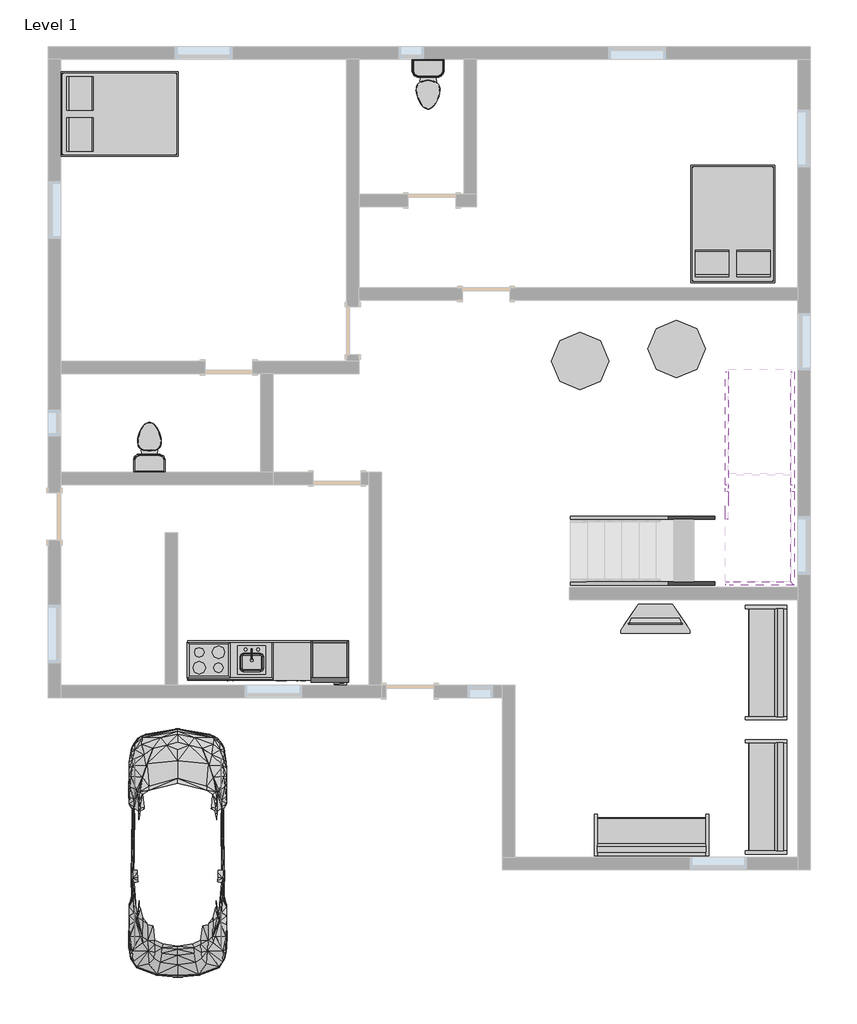
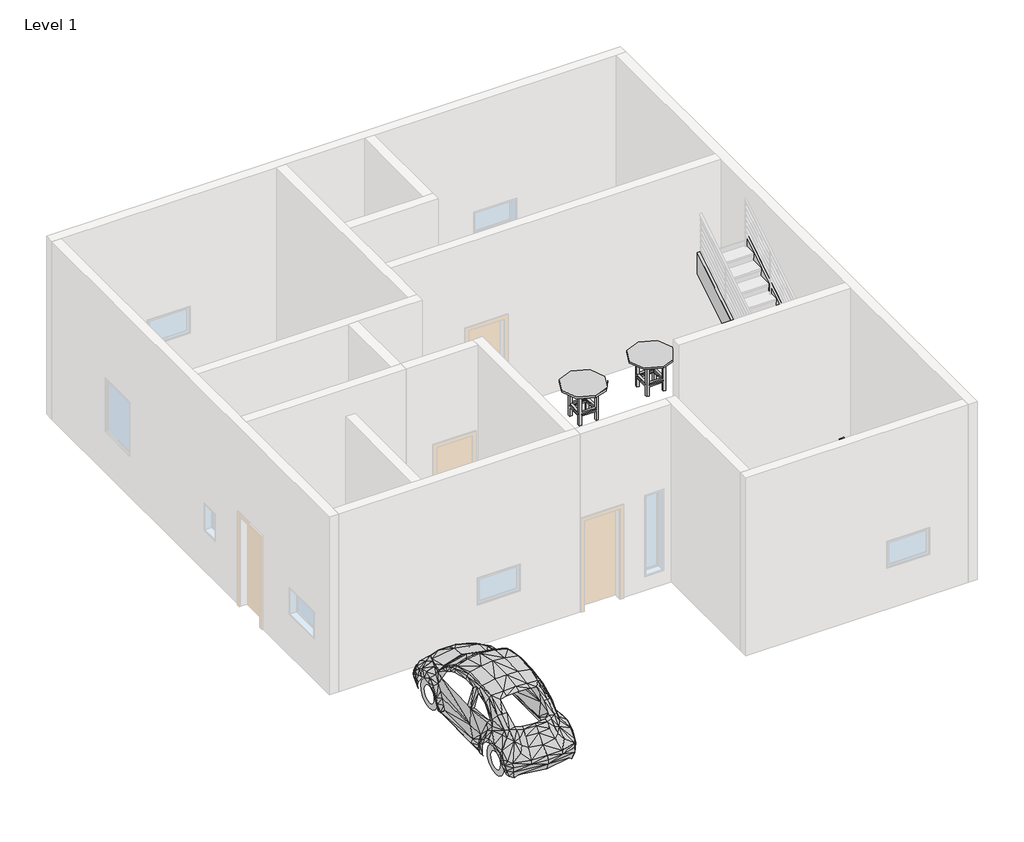
# One storey, part 4 of 4: 10 furniture elements, 7 members, 5 proxies, 3 flow terminals.
"""IFC4 building model written with IfcOpenShell, lengths in millimetres."""

from ifc_helpers import new_model, si_unit, frame, origin, place, context, project, spatial, polyline, outline, extrude, faceted_brep, transform, mapped, element, save
from components import m_cook_top_4_unit2_0615_x_500mm_249f3515, m_dishwasher_610_x_610_x_875mm_54ecfc4c, m_kitchenette_medium_1372mm_e05c6bec, m_rpc_beetle_m_rpc_beetle_b6d71803, m_refrigerator_600_x_660mm_a466bf94, m_sink_kitchen_island_450_x_450mm_f969cf2d, m_toilet_domestic_3d_m_toilet_domestic_3d_5cb52bd4, m_toilet_domestic_3d_m_toilet_domestic_3d_183bbd19, furniture_40ec15d9, furniture_0810mm_56245f3a, m_bed_box_1346_x_1880mm_double_b32eb57e, m_counter_top_w_sink_hole_600mm_depth_0a237b63, m_sofa_1830mm_f9e8a66b, m_table_dining_round_w_chairs_0915mm_diameter_5defa876

model = new_model("IFC4")

# Units and contexts
model_context = context("Model", 3, world=origin())
ifc_project = project(units=[si_unit("LENGTHUNIT", "METRE", prefix="MILLI")], contexts=[model_context])

# Site, building, storey
site = spatial("IfcSite", under=ifc_project)
building = spatial("IfcBuilding", under=site)
storey = spatial("IfcBuildingStorey", under=building, Name="Level 1", Elevation=0.0)

# Proxies
placement = place(None, origin())
m_cook_top_4_unit2_0615_x_500mm_shape = m_cook_top_4_unit2_0615_x_500mm_249f3515(model_context)
element("IfcBuildingElementProxy", 1, Name="M_Cook Top-4 Unit2 : 0615 x 500mm", ObjectType="M_Cook Top-4 Unit2 : 0615 x 500mm", at=placement, inside=storey, context=model_context, shape_type="MappedRepresentation", body=[
    mapped(m_cook_top_4_unit2_0615_x_500mm_shape, transform((-6183.3732634, 1498.698464, 0.0), x_axis=(1.0, 0.0, 0.0), y_axis=(0.0, 1.0, 0.0), z_axis=(0.0, 0.0, 1.0))),
])
m_dishwasher_610_x_610_x_875mm_shape = m_dishwasher_610_x_610_x_875mm_54ecfc4c(model_context)
element("IfcBuildingElementProxy", 2, Name="M_Dishwasher : 610 x 610 x 875mm", ObjectType="M_Dishwasher : 610 x 610 x 875mm", at=placement, inside=storey, context=model_context, shape_type="MappedRepresentation", body=[
    mapped(m_dishwasher_610_x_610_x_875mm_shape, transform((-5233.8907319, 1232.0488992, 0.0), x_axis=(1.0, 0.0, 0.0), y_axis=(0.0, 1.0, 0.0), z_axis=(0.0, 0.0, 1.0))),
])
m_kitchenette_medium_1372mm_shape = m_kitchenette_medium_1372mm_e05c6bec(model_context)
element("IfcBuildingElementProxy", 3, Name="M_Kitchenette - Medium : 1372mm", ObjectType="M_Kitchenette - Medium : 1372mm", at=placement, inside=storey, context=model_context, shape_type="MappedRepresentation", body=[
    mapped(m_kitchenette_medium_1372mm_shape, transform((-5859.1109683, 1803.698464, 0.0), x_axis=(1.0, 0.0, 0.0), y_axis=(0.0, 1.0, 0.0), z_axis=(0.0, 0.0, 1.0))),
])
m_rpc_beetle_m_rpc_beetle_shape = m_rpc_beetle_m_rpc_beetle_b6d71803(model_context)
element("IfcBuildingElementProxy", 4, Name="M_RPC Beetle : M_RPC Beetle", ObjectType="M_RPC Beetle : M_RPC Beetle", at=placement, inside=storey, context=model_context, shape_type="MappedRepresentation", body=[
    mapped(m_rpc_beetle_m_rpc_beetle_shape, transform((-6679.9732634, -2820.751536, 0.0), x_axis=(1.0, 0.0, 0.0), y_axis=(0.0, 1.0, 0.0), z_axis=(0.0, 0.0, 1.0))),
])
m_refrigerator_600_x_660mm_shape = m_refrigerator_600_x_660mm_a466bf94(model_context)
element("IfcBuildingElementProxy", 5, Name="M_Refrigerator : 600 x 660mm", ObjectType="M_Refrigerator : 600 x 660mm", at=placement, inside=storey, context=model_context, shape_type="MappedRepresentation", body=[
    mapped(m_refrigerator_600_x_660mm_shape, transform((-4192.5721207, 1507.4833738, 0.0), x_axis=(1.0, 0.0, 0.0), y_axis=(0.0, 1.0, 0.0), z_axis=(0.0, 0.0, 1.0))),
])

# Flow terminals
m_sink_kitchen_island_450_x_450mm_shape = m_sink_kitchen_island_450_x_450mm_f969cf2d(model_context)
element("IfcFlowTerminal", 6, ObjectType="M_Sink Kitchen-Island : 450 x 450mm", at=placement, inside=storey, context=model_context, shape_type="MappedRepresentation", body=[
    mapped(m_sink_kitchen_island_450_x_450mm_shape, transform((-5513.062504, 1496.3530629, 0.0), x_axis=(1.0, 0.0, 0.0), y_axis=(0.0, 1.0, 0.0), z_axis=(0.0, 0.0, 1.0))),
])
m_toilet_domestic_3d_m_toilet_domestic_3d_shape = m_toilet_domestic_3d_m_toilet_domestic_3d_5cb52bd4(model_context)
m_toilet_domestic_3d_m_toilet_domestic_3d_2_shape = m_toilet_domestic_3d_m_toilet_domestic_3d_183bbd19(model_context)
element("IfcFlowTerminal", 7, ObjectType="M_Toilet-Domestic-3D : M_Toilet-Domestic-3D", at=placement, inside=storey, context=model_context, shape_type="MappedRepresentation", body=[
    mapped(m_toilet_domestic_3d_m_toilet_domestic_3d_shape, transform((-7133.3692907, 4995.5444913, 0.0), x_axis=(-1.0, 0.0, 0.0), y_axis=(0.0, -1.0, 0.0), z_axis=(0.0, 0.0, 1.0))),
    mapped(m_toilet_domestic_3d_m_toilet_domestic_3d_2_shape, transform((-7133.3692907, 4995.5444913, 0.0), x_axis=(-1.0, 0.0, 0.0), y_axis=(0.0, -1.0, 0.0), z_axis=(0.0, 0.0, 1.0))),
])
element("IfcFlowTerminal", 8, ObjectType="M_Toilet-Domestic-3D : M_Toilet-Domestic-3D", at=placement, inside=storey, context=model_context, shape_type="MappedRepresentation", body=[
    mapped(m_toilet_domestic_3d_m_toilet_domestic_3d_shape, transform((-2677.5646035, 10610.1524366, 0.0), x_axis=(1.0, 0.0, 0.0), y_axis=(0.0, 1.0, 0.0), z_axis=(0.0, 0.0, 1.0))),
    mapped(m_toilet_domestic_3d_m_toilet_domestic_3d_2_shape, transform((-2677.5646035, 10610.1524366, 0.0), x_axis=(1.0, 0.0, 0.0), y_axis=(0.0, 1.0, 0.0), z_axis=(0.0, 0.0, 1.0))),
])

# Furniture
furniture_shape = furniture_40ec15d9(model_context)
element("IfcFurniture", 9, at=placement, inside=storey, context=model_context, shape_type="MappedRepresentation", body=[
    mapped(furniture_shape, transform((832.4258439, 2387.898464, 0.0), x_axis=(1.0, 0.0, 0.0), y_axis=(0.0, 1.0, 0.0), z_axis=(0.0, 0.0, 1.0))),
])
furniture_0810mm_shape = furniture_0810mm_56245f3a(model_context)
element("IfcFurniture", 10, ObjectType="0810mm", at=placement, inside=storey, context=model_context, shape_type="MappedRepresentation", body=[
    mapped(furniture_0810mm_shape, transform((961.5583601, 2138.8495806, 0.0), x_axis=(1.0, 0.0, 0.0), y_axis=(0.0, 1.0, 0.0), z_axis=(0.0, 0.0, 1.0))),
])
m_bed_box_1346_x_1880mm_double_shape = m_bed_box_1346_x_1880mm_double_b32eb57e(model_context)
element("IfcFurniture", 11, ObjectType="M_Bed-Box : 1346 x 1880mm - Double", at=placement, inside=storey, context=model_context, shape_type="MappedRepresentation", body=[
    mapped(m_bed_box_1346_x_1880mm_double_shape, transform((-7849.2027716, 9887.896005, 0.0), x_axis=(0.0, 1.0, 0.0), y_axis=(-1.0, 0.0, 0.0), z_axis=(0.0, 0.0, 1.0))),
])
element("IfcFurniture", 12, ObjectType="M_Bed-Box : 1346 x 1880mm - Double", at=placement, inside=storey, context=model_context, shape_type="MappedRepresentation", body=[
    mapped(m_bed_box_1346_x_1880mm_double_shape, transform((2536.3791956, 8233.0189558, 0.0), x_axis=(-1.0, 0.0, 0.0), y_axis=(0.0, -1.0, 0.0), z_axis=(0.0, 0.0, 1.0))),
])
m_counter_top_w_sink_hole_600mm_depth_shape = m_counter_top_w_sink_hole_600mm_depth_0a237b63(model_context)
element("IfcFurniture", 13, ObjectType="M_Counter Top w Sink Hole : 600mm Depth", at=placement, inside=storey, context=model_context, shape_type="MappedRepresentation", body=[
    mapped(m_counter_top_w_sink_hole_600mm_depth_shape, transform((-5325.9109683, 1803.698464, 0.0), x_axis=(1.0, 0.0, 0.0), y_axis=(0.0, 1.0, 0.0), z_axis=(0.0, 0.0, 1.0))),
])
m_sofa_1830mm_shape = m_sofa_1830mm_f9e8a66b(model_context)
element("IfcFurniture", 14, ObjectType="M_Sofa : 1830mm", at=placement, inside=storey, context=model_context, shape_type="MappedRepresentation", body=[
    mapped(m_sofa_1830mm_shape, transform((2581.4726382, 1526.4189558, 0.0), x_axis=(0.0, -0.9999999999999999, 0.0), y_axis=(0.9999999999999999, 0.0, 0.0), z_axis=(0.0, 0.0, 1.0))),
])
element("IfcFurniture", 15, ObjectType="M_Sofa : 1830mm", at=placement, inside=storey, context=model_context, shape_type="MappedRepresentation", body=[
    mapped(m_sofa_1830mm_shape, transform((2581.4726382, -616.7810442, 0.0), x_axis=(0.0, -1.0, 0.0), y_axis=(1.0, 0.0, 0.0), z_axis=(0.0, 0.0, 1.0))),
])
element("IfcFurniture", 16, ObjectType="M_Sofa : 1830mm", at=placement, inside=storey, context=model_context, shape_type="MappedRepresentation", body=[
    mapped(m_sofa_1830mm_shape, transform((969.1972284, -1150.5974377, 0.0), x_axis=(-1.0000000000000004, 0.0, 0.0), y_axis=(0.0, -1.0000000000000004, 0.0), z_axis=(0.0, 0.0, 1.0))),
])
m_table_dining_round_w_chairs_0915mm_diameter_shape = m_table_dining_round_w_chairs_0915mm_diameter_5defa876(model_context)
element("IfcFurniture", 17, ObjectType="M_Table-Dining Round w Chairs : 0915mm Diameter", at=placement, inside=storey, context=model_context, shape_type="MappedRepresentation", body=[
    mapped(m_table_dining_round_w_chairs_0915mm_diameter_shape, transform((-349.4250983, 6462.1271525, 0.0), x_axis=(1.0, 0.0, 0.0), y_axis=(0.0, 1.0, 0.0), z_axis=(0.0, 0.0, 1.0))),
])
element("IfcFurniture", 18, ObjectType="M_Table-Dining Round w Chairs : 0915mm Diameter", at=placement, inside=storey, context=model_context, shape_type="MappedRepresentation", body=[
    mapped(m_table_dining_round_w_chairs_0915mm_diameter_shape, transform((1193.5913431, 6656.0887971, 0.0), x_axis=(1.0, 0.0, 0.0), y_axis=(0.0, 1.0, 0.0), z_axis=(0.0, 0.0, 1.0))),
])

# Members
element("IfcMember", 19, ObjectType="Stringer - 50mm Width", at=placement, inside=storey, context=model_context, shape_type="SweptSolid", body=[
    extrude(outline(polyline([(215.089535, -399.786154), (0.0, -399.786154), (0.0, 8.4725788), (1307.5359792, 2076.013846), (1780.8128552, 2076.013846), (215.089535, -399.786154)])), frame((0.0, 3747.052048, 0.0), z_axis=(0.0, 1.0, 0.0), x_axis=(0.0, 0.0, 1.0)), (0.0, 0.0, 1.0), 50.0),
])
element("IfcMember", 20, ObjectType="Stringer - 50mm Width", at=placement, inside=storey, context=model_context, shape_type="SweptSolid", body=[
    extrude(outline(polyline([(215.089535, -399.786154), (0.0, -399.786154), (0.0, 8.4725788), (1386.5241617, 2200.9139095), (1786.5241617, 2085.0448495), (215.089535, -399.786154)])), frame((0.0, 2697.0262668, 0.0), z_axis=(0.0, 1.0, 0.0), x_axis=(0.0, 0.0, 1.0)), (0.0, 0.0, 1.0), 50.0),
])
element("IfcMember", 21, ObjectType="Stringer - 50mm Width", at=placement, inside=storey, context=model_context, shape_type="SweptSolid", body=[
    extrude(outline(polyline([(4303.9485275, 1386.5241617), (4188.0794675, 1786.5241617), (6103.248464, 2997.6982306), (6103.248464, 2524.4213547), (4303.9485275, 1386.5241617)])), frame((2076.013846, 0.0, 0.0), z_axis=(1.0, 0.0, 0.0), x_axis=(0.0, 1.0, 0.0)), (0.0, 0.0, 1.0), 50.0),
])
element("IfcMember", 22, ObjectType="Stringer - 50mm Width", at=placement, inside=storey, context=model_context, shape_type="SweptSolid", body=[
    extrude(outline(polyline([(4303.9485275, 1386.5241617), (4188.0794675, 1786.5241617), (6103.248464, 2997.6982306), (6103.248464, 2524.4213547), (4303.9485275, 1386.5241617)])), frame((3126.0396272, 0.0, 0.0), z_axis=(1.0, 0.0, 0.0), x_axis=(0.0, 1.0, 0.0)), (0.0, 0.0, 1.0), 50.0),
])
element("IfcMember", 23, ObjectType="Stringer - 50mm Width", at=placement, inside=storey, context=model_context, shape_type="SweptSolid", body=[
    extrude(outline(polyline([(4188.0794675, 1786.5241617), (4303.9485275, 1386.5241617), (3747.052048, 1386.5241617), (3747.052048, 1786.5241617), (4188.0794675, 1786.5241617)])), frame((2076.013846, 0.0, 0.0), z_axis=(1.0, 0.0, 0.0), x_axis=(0.0, 1.0, 0.0)), (0.0, 0.0, 1.0), 50.0),
])
element("IfcMember", 24, ObjectType="Stringer - 50mm Width", at=placement, inside=storey, context=model_context, shape_type="Brep", body=[
    faceted_brep([(2085.0448495, 2747.0262668, 1786.5241617), (2085.0448495, 2697.0262668, 1786.5241617), (3176.0396272, 2697.0262668, 1786.5241617), (3126.0396272, 2747.0262668, 1786.5241617), (2200.9139095, 2747.0262668, 1386.5241617), (3126.0396272, 2747.0262668, 1386.5241617), (2200.9139095, 2697.0262668, 1386.5241617), (3176.0396272, 2697.0262668, 1386.5241617)], [[[0, 1, 2, 3]], [[4, 0, 3, 5]], [[6, 4, 5, 7]], [[1, 6, 7, 2]], [[1, 0, 4, 6]], [[2, 7, 5, 3]]]),
])
element("IfcMember", 25, ObjectType="Stringer - 50mm Width", at=placement, inside=storey, context=model_context, shape_type="Brep", body=[
    faceted_brep([(3126.0396272, 2747.0262668, 1786.5241617), (3176.0396272, 2697.0262668, 1786.5241617), (3176.0396272, 4188.0794675, 1786.5241617), (3126.0396272, 4188.0794675, 1786.5241617), (3126.0396272, 2747.0262668, 1386.5241617), (3126.0396272, 4303.9485275, 1386.5241617), (3176.0396272, 2697.0262668, 1386.5241617), (3176.0396272, 4303.9485275, 1386.5241617)], [[[0, 1, 2, 3]], [[4, 0, 3, 5]], [[6, 4, 5, 7]], [[1, 6, 7, 2]], [[1, 0, 4, 6]], [[2, 7, 5, 3]]]),
])

save(model, "model.ifc")

# Revit data of these elements
# Type "M_Cook Top-4 Unit2 : 0615 x 500mm"
#   Depth = 1' - 7.68504"
#   Width = 2' - 0.2126"
#   Burner Material = Steel, Chrome Plated
#   Cooktop Material = Steel, Polished
#   Default Elevation = 0
#   Assembly Code = ""
# Type "M_Dishwasher : 610 x 610 x 875mm"
#   Label = "DW"
#   Depth = 2' - 0.01575"
#   Height = 2' - 10.44882"
#   Width = 2' - 0.01575"
#   Dishwasher Material = Steel, Paint Finish, Ivory, Glossy
#   Panel Face Material = Plastic, Opaque Black
#   Default Elevation = 0
# Type "M_Kitchenette - Medium : 1372mm"
#   Counter Length = 6' - 5.95276"
#   Cabinet Width = 4' - 6.01575"
#   Cabinet Height = 2' - 11.43307"
#   Cabinet Depth = 2' - 0.01575"
#   Toe Depth = 0' - 1.37795"
#   Toe Height = 0' - 3.93701"
#   Cabinet Material = Cabinets
#   Door/Drawer Material = Cabinets
#   Handle Material = Cabinets - Handles
#   Default Elevation = 0
# Type "M_RPC Beetle : M_RPC Beetle"
#   built-in parameter 1005198 = "{2, 15},{39, RPC-16-0U6E-L4EG-ENH1-J3KF-SVEL-0TX4-C0},{1, 0},{1, 0},{2, 18},{1, 8},{5, Color},{1, 0},{1, 0},{3, 0.8},{3, 0.8},{3, 0.8},{1, 8},{7, BBoxMin},{1, 0},{1, 0},{1, 0},{1, 0},{1, 0},{1, 8},{7, BBoxMax},{1, 0},{1, 0},{1, 0},{1, 0},{1, 0},{2, 11},{9, RPCTypeId},{1, 0},{1, 0},{39, RPC-16-0U6E-L4EG-ENH1-J3KF-SVEL-0TX4-C0},{1, 6},{14, RPCPlantHeight},{1, 0},{1, 0},{4, 4.92},{2, 11},{7, keyword},{1, 0},{1, 0},{39, :RPCs:Auto_Economy/Midsize:Geometry:RPC},{2, 11},{8, category},{1, 0},{1, 0},{20, Auto_Economy/Midsize},{2, 11},{12, LocalizedUID},{1, 0},{1, 0},{13, VW Beetle [4]},{2, 14},{6, Height},{1, 0},{1, 0},{4, 4.92},{1, 2},{16, Cast Reflections},{1, 0},{1, 0},{1, 0},{1, 4},{12, Transparency},{1, 0},{1, 0},{2, 18},{1, 4},{7, Tinting},{1, 0},{1, 0},{2, 50},{1, 2},{11, Use Tinting},{1, 0},{1, 0},{1, 0},{1, 2},{13, License Plate},{1, 0},{1, 0},{1, 0},{2, 11},{21, License Plate Texture},{1, 0},{1, 0},{64, __RPC:/object data/textures/car/plate/textures/default/rgb/0/0/0},{2, 11},{23, i_License Plate Texture},{1, 0},{1, 0},{0, },{1, 2},{12, Custom Plate},{1, 0},{1, 0},{1, 0},{2, 11},{23, License Plate File Name},{1, 0},{1, 0},{0, },{21, assetlibrary_base.fbx},{1, 5},"
#   built-in parameter 1005195 = "RPC-16-0U6E-L4EG-ENH1-J3KF-SVEL-0TX4-C0"
#   Height = 0
# Type "M_Refrigerator : 600 x 660mm"
#   Label = "REF."
#   Depth = 2' - 1.98425"
#   Height = 6' - 0.04724"
#   Width = 1' - 11.62205"
#   Material = Steel, Paint Finish, Ivory, Matte
#   Description = (empty or 0)
#   Default Elevation = 0
# Type "M_Sink Kitchen-Island : 450 x 450mm"
#   Counter Height [instance default] = 2' - 11.43307"
#   Depth = 1' - 5.71654"
#   Width = 1' - 5.71654"
#   Fixture Material = Steel, Polished
#   Sink Material = Steel, Polished
#   Default Elevation = 0
# Type "M_Toilet-Domestic-3D : M_Toilet-Domestic-3D"
#   Bowl/Basin Material = Porcelain, Linen
#   Seat Material = Laminate, Linen, Matte
#   Default Elevation = 0
# Type
#   Depth = 1' - 6.11024"
#   Width = 3' - 7.30709"
#   Height = 1' - 7.68504"
#   Finish = Melamine - Gray
#   Default Elevation = 0
# Type "0810mm"
#   SinAng = 0' - 0.0193"
#   L = 2' - 3.79372"
#   H = 1' - 3.6354"
#   Thickness = 0' - 4.33071"
#   Diagonal = 2' - 7.88976"
#   CosAng = 0' - 0.03431"
#   Stand [instance default] = yes
#   Default Elevation = 0
# Type "M_Bed-Box : 1346 x 1880mm - Double"
#   Length = 6' - 2.01575"
#   Width = 4' - 4.99213"
#   Frame Material = Birch
#   Mattress Material = Linen, White
#   Default Elevation = 0
# Type "M_Counter Top w Sink Hole : 600mm Depth"
#   Counter Thickness = 0' - 1.5748"
#   Depth = 2' - 0.6063"
#   Height = 2' - 11.43307"
#   Length [instance default] = 8' - 2.4252"
#   Sink Location [instance default] = 3' - 11.24409"
#   Sink Location To Wall [instance default] = 0' - 3.93701"
#   Sink Opening Depth [instance default] = 1' - 2.88189"
#   Sink Opening Width [instance default] = 1' - 11.11024"
#   Counter Top Material = none
#   Default Elevation = 0
# Type "M_Sofa : 1830mm"
#   Width = 6' - 0.04724"
#   Seat Material = Linen, Beige
#   Frame Material = Cherry
#   Default Elevation = 0
# Type "M_Table-Dining Round w Chairs : 0915mm Diameter"
#   Radius = 1' - 6.01181"
#   Diameter = 3' - 0.02362"
#   Height = 2' - 6"
#   Chairs = 4
#   Base Material = Pine
#   Top Material = Laminate, Linen, Matte
#   Default Elevation = 0
# Element 1 (IfcBuildingElementProxy, "M_Cook Top-4 Unit2 : 0615 x 500mm")
#   Phase Created = New Construction
#   Materials on its faces: "Steel, Polished", "Steel, Chrome Plated"
# Element 2 (IfcBuildingElementProxy, "M_Dishwasher : 610 x 610 x 875mm")
#   Phase Created = New Construction
#   Materials on its faces: "Steel, Paint Finish, Ivory, Glossy", "Plastic, Opaque Black"
# Element 3 (IfcBuildingElementProxy, "M_Kitchenette - Medium : 1372mm")
#   Phase Created = New Construction
#   Materials on its faces: "Cabinets", "Cabinets - Handles"
# Element 4 (IfcBuildingElementProxy, "M_RPC Beetle : M_RPC Beetle")
#   Phase Created = New Construction
# Element 5 (IfcBuildingElementProxy, "M_Refrigerator : 600 x 660mm")
#   Phase Created = New Construction
#   Materials on its faces: "Steel, Paint Finish, Ivory, Matte", "Steel, Chrome Plated"
# Element 6 (IfcFlowTerminal, "M_Sink Kitchen-Island : 450 x 450mm")
#   Mark = "3"
#   Counter Height = 2' - 11.43307"
#   Phase Created = New Construction
#   Materials on its faces: "Steel, Polished"
# Element 7 (IfcFlowTerminal, "M_Toilet-Domestic-3D : M_Toilet-Domestic-3D")
#   Mark = "1"
#   Phase Created = New Construction
#   Materials on its faces: "Porcelain, Linen", "Laminate, Linen, Matte"
# Element 8 (IfcFlowTerminal, "M_Toilet-Domestic-3D : M_Toilet-Domestic-3D")
#   Mark = "2"
#   Phase Created = New Construction
#   Materials on its faces: "Porcelain, Linen", "Laminate, Linen, Matte"
# Element 9 (IfcFurniture)
#   Phase Created = New Construction
#   Materials on its faces: "Melamine - Gray", "Glass - Shelves"
# Element 10 (IfcFurniture, "0810mm")
#   Stand = yes
#   Phase Created = New Construction
#   Materials on its faces: "TV - Black", "TV - Glass", "TV - Screen"
# Elements 11, 12 (IfcFurniture, "M_Bed-Box : 1346 x 1880mm - Double")
#   Phase Created = New Construction
#   Materials on its faces: "Birch", "Linen, White"
# Element 13 (IfcFurniture, "M_Counter Top w Sink Hole : 600mm Depth")
#   Sink Opening Width = 1' - 3.74803"
#   Sink Opening Depth = 1' - 1.77953"
#   Sink Location To Wall = 0' - 6.29921"
#   Sink Location = 3' - 4.35433"
#   Length = 6' - 5.95276"
#   Phase Created = New Construction
#   Materials on its faces: "Counter Top"
# Elements 14, 15, 16 (IfcFurniture, "M_Sofa : 1830mm")
#   Phase Created = New Construction
#   Materials on its faces: "Cherry", "Linen, Beige"
# Elements 17, 18 (IfcFurniture, "M_Table-Dining Round w Chairs : 0915mm Diameter")
#   Phase Created = New Construction
#   Materials on its faces: "Pine", "Laminate, Linen, Matte"
# Elements 19, 20, 21, 22, 23, 24, 25 (IfcMember, "Stringer - 50mm Width")
#   Phase Created = New Construction
# Materials
#   "Steel, Chrome Plated": class "Metal", colour RGB 244 244 244, transparency 0, Description = "Chromiuim plated steel", Cost = 0
#   "Steel, Polished": class "Metal", colour RGB 57 57 57, transparency 0, Description = "Polished steel", Cost = 0
#   "Steel, Paint Finish, Ivory, Glossy": class "Metal", colour RGB 247 247 239, transparency 0, Description = "Steel, paint finish, ivory, glossy", Cost = 0
#   "Plastic, Opaque Black": class "Plastic", colour RGB 0 0 0, transparency 0.7, Description = "Plastic, generic, opaque black", Cost = 0
#   "Cabinets": colour RGB 249 249 249, transparency 0
#   "Cabinets - Handles": class "Metal", colour RGB 57 57 57, transparency 0
#   "Steel, Paint Finish, Ivory, Matte": class "Metal", colour RGB 247 247 239, transparency 0, Description = "Steel, paint finish, ivory, matte", Cost = 0
#   "Porcelain, Linen": class "Ceramic", colour RGB 249 239 230, transparency 0, Description = "Porcelain, linen", Cost = 0
#   "Laminate, Linen, Matte": class "Plastic", colour RGB 249 239 230, transparency 0, Description = "Plastic Laminate - Linen, Matte", Cost = 0
#   "Melamine - Gray": class "Wood", colour RGB 49 49 49, transparency 0
#   "Birch": class "Wood", colour RGB 224 178 126, transparency 0, Description = "Betula Alleghaniensis", Cost = 0
#   "Linen, White": class "Textile", colour RGB 247 247 239, transparency 0, Description = "Linen, white", Cost = 0
#   "Linen, Beige": class "Textile", colour RGB 249 239 230, transparency 0, Description = "Linen, beige", Cost = 0
#   "Cherry": class "Wood", colour RGB 154 107 61, transparency 0, Description = "Prunus Serotina", Cost = 0
#   "Pine": class "Wood", colour RGB 223 192 134, transparency 0, Description = "Pinus Echinata", Cost = 0
#   "Glass - Shelves": class "Glass", colour RGB 167 167 167, transparency 0.9
#   "TV - Black": colour RGB 49 49 49, transparency 0
#   "TV - Glass": colour RGB 157 157 157, transparency 0.9
#   "TV - Screen": colour RGB 0 0 0, transparency 0
#   "Counter Top": class "Wood", colour RGB 226 177 128, transparency 0
